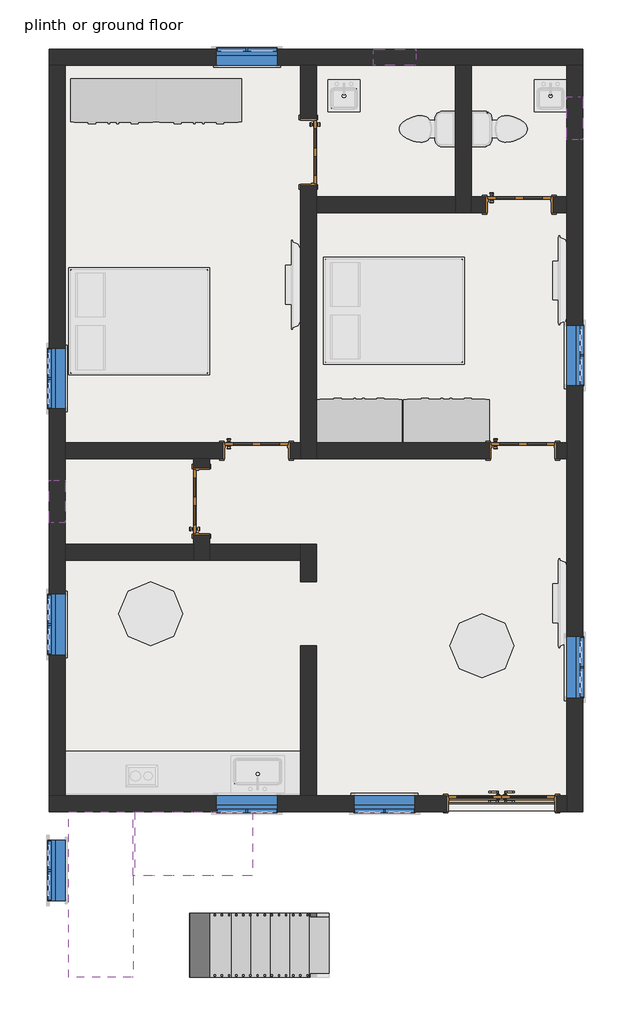
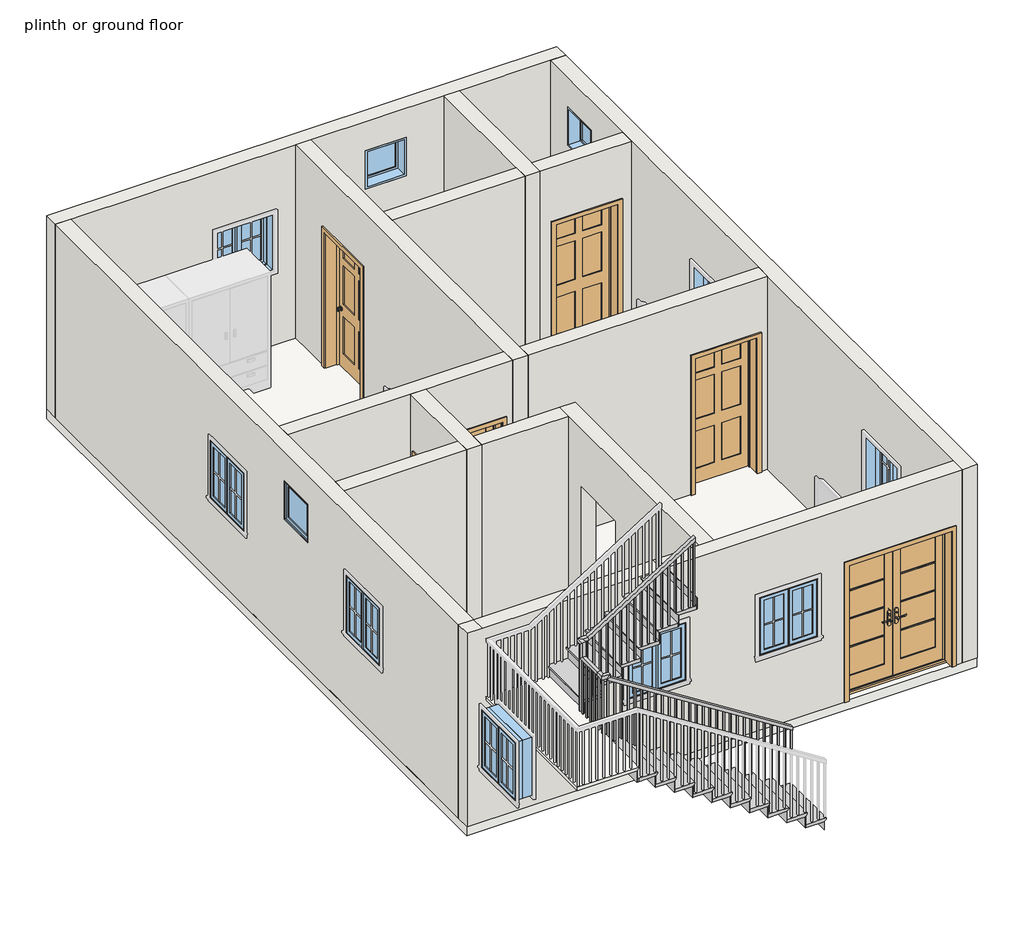
# One storey, part 1 of 3: 14 walls, 11 windows, 6 doors, 2 slabs, 2 stair flights, 1 railing.
# Revit data of these elements (continued)
# Element 36 (IfcWindow, "Window-Casement-Double : 34\" x 36\"")
#   Mark = "39"
#   Window Inset = 0' - 0"
#   Interior Wall Closure = 0' - 2 1/4"
#   Frame Extension = 0' - 0 1/4"
#   Exterior Wall Closure = 0' - 1 1/4"
#   Interior Trim Visibility = yes
#   Exterior Trim Visibility = yes
#   Phase Created = New Construction
#   Materials on its faces: "Wood - Stained", "Glass", "Clad - White"
# Materials
#   "Cherry": class "Wood", colour RGB 226 177 128, transparency 0, Description = "Prunus Serotina", Cost = 0
#   "Glass": class "Glass", colour RGB 0 128 192, transparency 0.75, Description = "Soda Lime Glass", Cost = 0
#   "Aluminum": class "Metal", colour RGB 247 247 247, transparency 0, Description = "Aluminum 6061", Cost = 0
#   "Concrete, Cast-in-Place gray": class "Concrete", colour RGB 192 192 192, transparency 0, Description = "Cast-in-place concrete", Cost = 0
#   "Sash": class "Wood", colour RGB 224 178 126, transparency 0, Cost = 0
#   "Wood - Stained": class "Wood", colour RGB 224 178 126, transparency 0, Cost = 0
#   "Clad - White": class "Wood", colour RGB 242 242 238, transparency 0, Cost = 0
#   "Laminate, Ivory, Matte": class "Plastic", colour RGB 247 247 239, transparency 0, Description = "Plastic Laminate - Ivory, Matte", Cost = 0
#   "Default Wall": colour RGB 128 128 128, transparency 0, Cost = 0
#   "Birch": class "Wood", colour RGB 224 178 126, transparency 0, Description = "Betula Alleghaniensis", Cost = 0
# Room at (20884.014, 14133.303) mm, phase "New Construction", upper level "plinth or ground floor", upper offset 10' - 0", lower offset 0' - 0"
#   Number = "1"
#   Name = "MASTER BED ROOM"
# Room at (24720.881, 14133.303) mm, phase "New Construction", upper level "plinth or ground floor", upper offset 10' - 0", lower offset 0' - 0"
#   Number = "2"
#   Name = "GUEST ROOM"
# Room at (24720.881, 8727.08) mm, phase "New Construction", upper level "plinth or ground floor", upper offset 10' - 0", lower offset 0' - 0"
#   Number = "3"
#   Name = "LIVING HALL"
# Room at (21178.516, 8306.363) mm, phase "New Construction", upper level "plinth or ground floor", upper offset 10' - 0", lower offset 0' - 0"
#   Number = "4"
#   Name = "KITCHEN, DINING"
# Room at (20189.83, 11272.423) mm, phase "New Construction", upper level "plinth or ground floor", upper offset 10' - 0", lower offset 0' - 0"
#   Number = "5"
# Room at (23702.823, 16558.841) mm, phase "New Construction", upper level "plinth or ground floor", upper offset 10' - 0", lower offset 0' - 0"
#   Number = "6"
#   Name = "TOILET"
# Room at (25898.891, 16558.841) mm, phase "New Construction", upper level "plinth or ground floor", upper offset 10' - 0", lower offset 0' - 0"
#   Number = "7"
#   Name = "TOILET"
# Room at (25133.263, 5024.765) mm, phase "New Construction", upper level "plinth or ground floor", upper offset 10' - 0", lower offset 0' - 0"
#   Number = "8"
#   Name = "ENTRANCE"
# Room, not placed, phase "New Construction", upper offset 0' - 0", lower offset 0' - 0"
#   Number = "9"
#   Name = "MASTER BED ROOM"
# Room, not placed, phase "New Construction", upper offset 0' - 0", lower offset 0' - 0"
#   Number = "10"
#   Name = "GUEST ROOM"
# Room, not placed, phase "New Construction", upper offset 0' - 0", lower offset 0' - 0"
#   Number = "11"
#   Name = "LIVING HALL"
# Room, not placed, phase "New Construction", upper offset 0' - 0", lower offset 0' - 0"
#   Number = "12"
#   Name = "KITCHEN, DINING"
# Room, not placed, phase "New Construction", upper offset 0' - 0", lower offset 0' - 0"
#   Number = "13"
# Room, not placed, phase "New Construction", upper offset 0' - 0", lower offset 0' - 0"
#   Number = "14"
#   Name = "TOILET"
# Room, not placed, phase "New Construction", upper offset 0' - 0", lower offset 0' - 0"
#   Number = "15"
#   Name = "TOILET"
# Room, not placed, phase "New Construction", upper offset 0' - 0", lower offset 0' - 0"
#   Number = "16"
#   Name = "ENTRANCE"
